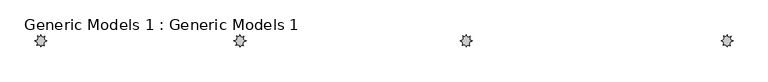
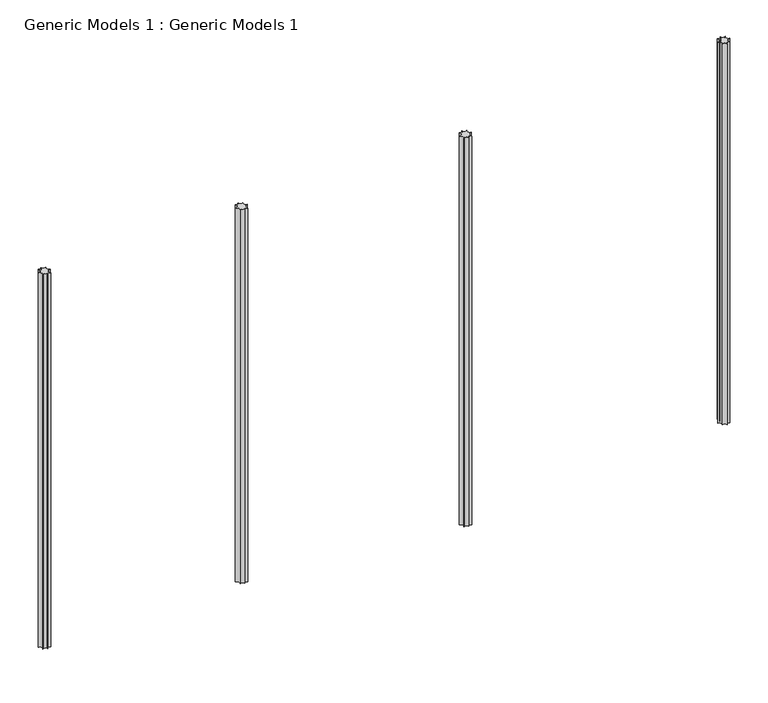
"""IFC4 building model written with IfcOpenShell, lengths in millimetres: proxy geometry, Generic Models 1 : Generic Models 1."""

from ifc_helpers import new_model, si_unit, frame, origin, place, context, project, spatial, polyline, circle_curve, source, transform, mapped, element, save
from ifc_brep_helpers import plane_surface, revolved_surface, advanced_brep


def generic_models_1_generic_models_1_27fef2d6(model_context):
    return source(origin(), model_context, "Body", "AdvancedBrep", [
        advanced_brep(
        [(-16868.2183666, -7371.697034, 6717.0608213), (-16912.6683666, -7455.6996381, 6717.0608213), (-16878.4321748, -7531.7567045, 6717.0608213), (-16811.0683666, -7557.2996381, 6717.0608213), (-16753.9183666, -7539.7022422, 6717.0608213), (-16709.4683666, -7455.6996381, 6717.0608213), (-16743.7045585, -7379.6425717, 6717.0608213), (-16811.0683666, -7354.0996381, 6717.0608213), (-16868.2183666, -7371.697034, 0.0), (-16811.0683666, -7354.0996381, 0.0), (-16743.7045585, -7379.6425717, 0.0), (-16709.4683666, -7455.6996381, 0.0), (-16753.9183666, -7539.7022422, 0.0), (-16811.0683666, -7557.2996381, 0.0), (-16878.4321748, -7531.7567045, 0.0), (-16912.6683666, -7455.6996381, 0.0)],
        [
            (0, 1, circle_curve(frame((-16912.6683666, -7401.9379714, 6717.0608213), z_axis=(0.0, 0.0, -1.0), x_axis=(1.0, 0.0, 0.0)), 53.7616666)),
            (1, 2, circle_curve(frame((-16912.6683666, -7501.4336804, 6717.0608213), z_axis=(0.0, 0.0, -1.0), x_axis=(1.0, 0.0, 0.0)), 45.7340423)),
            (2, 3, circle_curve(frame((-16849.5929412, -7557.2996381, 6717.0608213), z_axis=(0.0, 0.0, -1.0), x_axis=(1.0, 0.0, 0.0)), 38.5245746)),
            (3, 4, circle_curve(frame((-16779.7841073, -7557.2996381, 6717.0608213), z_axis=(0.0, 0.0, -1.0), x_axis=(1.0, 0.0, 0.0)), 31.2842593)),
            (4, 5, circle_curve(frame((-16709.4683666, -7509.4613047, 6717.0608213), z_axis=(0.0, 0.0, -1.0), x_axis=(1.0, 0.0, 0.0)), 53.7616666)),
            (5, 6, circle_curve(frame((-16709.4683666, -7409.9655958, 6717.0608213), z_axis=(0.0, 0.0, -1.0), x_axis=(1.0, 0.0, 0.0)), 45.7340423)),
            (6, 7, circle_curve(frame((-16772.543792, -7354.0996381, 6717.0608213), z_axis=(0.0, 0.0, -1.0), x_axis=(1.0, 0.0, 0.0)), 38.5245746)),
            (7, 0, circle_curve(frame((-16842.352626, -7354.0996381, 6717.0608213), z_axis=(0.0, 0.0, -1.0), x_axis=(1.0, 0.0, 0.0)), 31.2842593)),
            (8, 9, circle_curve(frame((-16842.352626, -7354.0996381, 0.0), z_axis=(0.0, 0.0, 1.0), x_axis=(1.0, 0.0, 0.0)), 31.2842593)),
            (9, 10, circle_curve(frame((-16772.543792, -7354.0996381, 0.0), z_axis=(0.0, 0.0, 1.0), x_axis=(1.0, 0.0, 0.0)), 38.5245746)),
            (10, 11, circle_curve(frame((-16709.4683666, -7409.9655958, 0.0), z_axis=(0.0, 0.0, 1.0), x_axis=(1.0, 0.0, 0.0)), 45.7340423)),
            (11, 12, circle_curve(frame((-16709.4683666, -7509.4613047, 0.0), z_axis=(0.0, 0.0, 1.0), x_axis=(1.0, 0.0, 0.0)), 53.7616666)),
            (12, 13, circle_curve(frame((-16779.7841073, -7557.2996381, 0.0), z_axis=(0.0, 0.0, 1.0), x_axis=(1.0, 0.0, 0.0)), 31.2842593)),
            (13, 14, circle_curve(frame((-16849.5929412, -7557.2996381, 0.0), z_axis=(0.0, 0.0, 1.0), x_axis=(1.0, 0.0, 0.0)), 38.5245746)),
            (14, 15, circle_curve(frame((-16912.6683666, -7501.4336804, 0.0), z_axis=(0.0, 0.0, 1.0), x_axis=(1.0, 0.0, 0.0)), 45.7340423)),
            (15, 8, circle_curve(frame((-16912.6683666, -7401.9379714, 0.0), z_axis=(0.0, 0.0, 1.0), x_axis=(1.0, 0.0, 0.0)), 53.7616666)),
            (0, 8),
            (15, 1),
            (14, 2),
            (13, 3),
            (12, 4),
            (11, 5),
            (10, 6),
            (9, 7),
        ],
        [
            plane_surface(frame((-16858.9067, -7401.9379714, 6717.0608213), z_axis=(0.0, 0.0, 1.0), x_axis=(0.0, -1.0, 0.0))),
            plane_surface(frame((-16858.9067, -7401.9379714, 0.0), z_axis=(0.0, 0.0, -1.0), x_axis=(0.0, 1.0, 0.0))),
            revolved_surface(polyline([(-16858.9067, -7401.9379714, 0.0), (-16858.9067, -7401.9379714, 6717.0608213)]), (-16912.6683666, -7401.9379714, 0.0), (0.0, 0.0, -1.0)),
            revolved_surface(polyline([(-16866.9343243, -7501.4336804, 0.0), (-16866.9343243, -7501.4336804, 6717.0608213)]), (-16912.6683666, -7501.4336804, 0.0), (0.0, 0.0, -1.0)),
            revolved_surface(polyline([(-16811.0683666, -7557.2996381, 0.0), (-16811.0683666, -7557.2996381, 6717.0608213)]), (-16849.5929412, -7557.2996381, 0.0), (0.0, 0.0, -1.0)),
            revolved_surface(polyline([(-16748.499848000003, -7557.2996381, 0.0), (-16748.499848000003, -7557.2996381, 6717.0608213)]), (-16779.7841073, -7557.2996381, 0.0), (0.0, 0.0, -1.0)),
            revolved_surface(polyline([(-16655.7067, -7509.4613047, 0.0), (-16655.7067, -7509.4613047, 6717.0608213)]), (-16709.4683666, -7509.4613047, 0.0), (0.0, 0.0, -1.0)),
            revolved_surface(polyline([(-16663.7343243, -7409.9655958, 0.0), (-16663.7343243, -7409.9655958, 6717.0608213)]), (-16709.4683666, -7409.9655958, 0.0), (0.0, 0.0, -1.0)),
            revolved_surface(polyline([(-16734.0192174, -7354.0996381, 0.0), (-16734.0192174, -7354.0996381, 6717.0608213)]), (-16772.543792, -7354.0996381, 0.0), (0.0, 0.0, -1.0)),
            revolved_surface(polyline([(-16811.0683667, -7354.0996381, 0.0), (-16811.0683667, -7354.0996381, 6717.0608213)]), (-16842.352626, -7354.0996381, 0.0), (0.0, 0.0, -1.0)),
        ],
        [
            (0, [[1, 2, 3, 4, 5, 6, 7, 8]]),
            (1, [[9, 10, 11, 12, 13, 14, 15, 16]]),
            (2, [[-1, 17, -16, 18]]),
            (3, [[-2, -18, -15, 19]]),
            (4, [[-3, -19, -14, 20]]),
            (5, [[-4, -20, -13, 21]]),
            (6, [[-5, -21, -12, 22]]),
            (7, [[-6, -22, -11, 23]]),
            (8, [[-7, -23, -10, 24]]),
            (9, [[-8, -24, -9, -17]]),
        ],
    ),
        advanced_brep(
        [(-13058.2183666, -7371.697034, 6680.2), (-13102.6683666, -7455.6996381, 6680.2), (-13068.4321748, -7531.7567045, 6680.2), (-13001.0683666, -7557.2996381, 6680.2), (-12943.9183666, -7539.7022422, 6680.2), (-12899.4683666, -7455.6996381, 6680.2), (-12933.7045585, -7379.6425717, 6680.2), (-13001.0683666, -7354.0996381, 6680.2), (-13058.2183666, -7371.697034, -309.3465665), (-13001.0683666, -7354.0996381, -309.3465665), (-12933.7045585, -7379.6425717, -309.3465665), (-12899.4683666, -7455.6996381, -309.3465665), (-12943.9183666, -7539.7022422, -309.3465665), (-13001.0683666, -7557.2996381, -309.3465665), (-13068.4321748, -7531.7567045, -309.3465665), (-13102.6683666, -7455.6996381, -309.3465665)],
        [
            (0, 1, circle_curve(frame((-13102.6683666, -7401.9379714, 6680.2), z_axis=(0.0, 0.0, -1.0), x_axis=(1.0, 0.0, 0.0)), 53.7616666)),
            (1, 2, circle_curve(frame((-13102.6683666, -7501.4336804, 6680.2), z_axis=(0.0, 0.0, -1.0), x_axis=(1.0, 0.0, 0.0)), 45.7340423)),
            (2, 3, circle_curve(frame((-13039.5929412, -7557.2996381, 6680.2), z_axis=(0.0, 0.0, -1.0), x_axis=(1.0, 0.0, 0.0)), 38.5245746)),
            (3, 4, circle_curve(frame((-12969.7841073, -7557.2996381, 6680.2), z_axis=(0.0, 0.0, -1.0), x_axis=(1.0, 0.0, 0.0)), 31.2842593)),
            (4, 5, circle_curve(frame((-12899.4683666, -7509.4613047, 6680.2), z_axis=(0.0, 0.0, -1.0), x_axis=(1.0, 0.0, 0.0)), 53.7616666)),
            (5, 6, circle_curve(frame((-12899.4683666, -7409.9655958, 6680.2), z_axis=(0.0, 0.0, -1.0), x_axis=(1.0, 0.0, 0.0)), 45.7340423)),
            (6, 7, circle_curve(frame((-12962.543792, -7354.0996381, 6680.2), z_axis=(0.0, 0.0, -1.0), x_axis=(1.0, 0.0, 0.0)), 38.5245746)),
            (7, 0, circle_curve(frame((-13032.352626, -7354.0996381, 6680.2), z_axis=(0.0, 0.0, -1.0), x_axis=(1.0, 0.0, 0.0)), 31.2842593)),
            (8, 9, circle_curve(frame((-13032.352626, -7354.0996381, -309.3465665), z_axis=(0.0, 0.0, 1.0), x_axis=(1.0, 0.0, 0.0)), 31.2842593)),
            (9, 10, circle_curve(frame((-12962.543792, -7354.0996381, -309.3465665), z_axis=(0.0, 0.0, 1.0), x_axis=(1.0, 0.0, 0.0)), 38.5245746)),
            (10, 11, circle_curve(frame((-12899.4683666, -7409.9655958, -309.3465665), z_axis=(0.0, 0.0, 1.0), x_axis=(1.0, 0.0, 0.0)), 45.7340423)),
            (11, 12, circle_curve(frame((-12899.4683666, -7509.4613047, -309.3465665), z_axis=(0.0, 0.0, 1.0), x_axis=(1.0, 0.0, 0.0)), 53.7616666)),
            (12, 13, circle_curve(frame((-12969.7841073, -7557.2996381, -309.3465665), z_axis=(0.0, 0.0, 1.0), x_axis=(1.0, 0.0, 0.0)), 31.2842593)),
            (13, 14, circle_curve(frame((-13039.5929412, -7557.2996381, -309.3465665), z_axis=(0.0, 0.0, 1.0), x_axis=(1.0, 0.0, 0.0)), 38.5245746)),
            (14, 15, circle_curve(frame((-13102.6683666, -7501.4336804, -309.3465665), z_axis=(0.0, 0.0, 1.0), x_axis=(1.0, 0.0, 0.0)), 45.7340423)),
            (15, 8, circle_curve(frame((-13102.6683666, -7401.9379714, -309.3465665), z_axis=(0.0, 0.0, 1.0), x_axis=(1.0, 0.0, 0.0)), 53.7616666)),
            (0, 8),
            (15, 1),
            (14, 2),
            (13, 3),
            (12, 4),
            (11, 5),
            (10, 6),
            (9, 7),
        ],
        [
            plane_surface(frame((-13048.9067, -7401.9379714, 6680.2), z_axis=(0.0, 0.0, 1.0), x_axis=(0.0, -1.0, 0.0))),
            plane_surface(frame((-13048.9067, -7401.9379714, -309.3465665), z_axis=(0.0, 0.0, -1.0), x_axis=(0.0, 1.0, 0.0))),
            revolved_surface(polyline([(-13048.906700000001, -7401.9379714, -309.3465665), (-13048.906700000001, -7401.9379714, 6680.2)]), (-13102.6683666, -7401.9379714, -309.3465665), (0.0, 0.0, -1.0)),
            revolved_surface(polyline([(-13056.9343243, -7501.4336804, -309.3465665), (-13056.9343243, -7501.4336804, 6680.2)]), (-13102.6683666, -7501.4336804, -309.3465665), (0.0, 0.0, -1.0)),
            revolved_surface(polyline([(-13001.0683666, -7557.2996381, -309.3465665), (-13001.0683666, -7557.2996381, 6680.2)]), (-13039.5929412, -7557.2996381, -309.3465665), (0.0, 0.0, -1.0)),
            revolved_surface(polyline([(-12938.499848, -7557.2996381, -309.3465665), (-12938.499848, -7557.2996381, 6680.2)]), (-12969.7841073, -7557.2996381, -309.3465665), (0.0, 0.0, -1.0)),
            revolved_surface(polyline([(-12845.7067, -7509.4613047, -309.3465665), (-12845.7067, -7509.4613047, 6680.2)]), (-12899.4683666, -7509.4613047, -309.3465665), (0.0, 0.0, -1.0)),
            revolved_surface(polyline([(-12853.7343243, -7409.9655958, -309.3465665), (-12853.7343243, -7409.9655958, 6680.2)]), (-12899.4683666, -7409.9655958, -309.3465665), (0.0, 0.0, -1.0)),
            revolved_surface(polyline([(-12924.0192174, -7354.0996381, -309.3465665), (-12924.0192174, -7354.0996381, 6680.2)]), (-12962.543792, -7354.0996381, -309.3465665), (0.0, 0.0, -1.0)),
            revolved_surface(polyline([(-13001.0683667, -7354.0996381, -309.3465665), (-13001.0683667, -7354.0996381, 6680.2)]), (-13032.352626, -7354.0996381, -309.3465665), (0.0, 0.0, -1.0)),
        ],
        [
            (0, [[1, 2, 3, 4, 5, 6, 7, 8]]),
            (1, [[9, 10, 11, 12, 13, 14, 15, 16]]),
            (2, [[-1, 17, -16, 18]]),
            (3, [[-2, -18, -15, 19]]),
            (4, [[-3, -19, -14, 20]]),
            (5, [[-4, -20, -13, 21]]),
            (6, [[-5, -21, -12, 22]]),
            (7, [[-6, -22, -11, 23]]),
            (8, [[-7, -23, -10, 24]]),
            (9, [[-8, -24, -9, -17]]),
        ],
    ),
        advanced_brep(
        [(-8664.0183666, -7371.697034, 6832.6), (-8708.4683666, -7455.6996381, 6832.6), (-8674.2321748, -7531.7567045, 6832.6), (-8606.8683666, -7557.2996381, 6832.6), (-8549.7183666, -7539.7022422, 6832.6), (-8505.2683666, -7455.6996381, 6832.6), (-8539.5045585, -7379.6425717, 6832.6), (-8606.8683666, -7354.0996381, 6832.6), (-8664.0183666, -7371.697034, -15.8978184), (-8606.8683666, -7354.0996381, -15.8978184), (-8539.5045585, -7379.6425717, -15.8978184), (-8505.2683666, -7455.6996381, -15.8978184), (-8549.7183666, -7539.7022422, -15.8978184), (-8606.8683666, -7557.2996381, -15.8978184), (-8674.2321748, -7531.7567045, -15.8978184), (-8708.4683666, -7455.6996381, -15.8978184)],
        [
            (0, 1, circle_curve(frame((-8708.4683666, -7401.9379714, 6832.6), z_axis=(0.0, 0.0, -1.0), x_axis=(1.0, 0.0, 0.0)), 53.7616666)),
            (1, 2, circle_curve(frame((-8708.4683666, -7501.4336804, 6832.6), z_axis=(0.0, 0.0, -1.0), x_axis=(1.0, 0.0, 0.0)), 45.7340423)),
            (2, 3, circle_curve(frame((-8645.3929412, -7557.2996381, 6832.6), z_axis=(0.0, 0.0, -1.0), x_axis=(1.0, 0.0, 0.0)), 38.5245746)),
            (3, 4, circle_curve(frame((-8575.5841073, -7557.2996381, 6832.6), z_axis=(0.0, 0.0, -1.0), x_axis=(1.0, 0.0, 0.0)), 31.2842593)),
            (4, 5, circle_curve(frame((-8505.2683666, -7509.4613047, 6832.6), z_axis=(0.0, 0.0, -1.0), x_axis=(1.0, 0.0, 0.0)), 53.7616666)),
            (5, 6, circle_curve(frame((-8505.2683666, -7409.9655958, 6832.6), z_axis=(0.0, 0.0, -1.0), x_axis=(1.0, 0.0, 0.0)), 45.7340423)),
            (6, 7, circle_curve(frame((-8568.343792, -7354.0996381, 6832.6), z_axis=(0.0, 0.0, -1.0), x_axis=(1.0, 0.0, 0.0)), 38.5245746)),
            (7, 0, circle_curve(frame((-8638.152626, -7354.0996381, 6832.6), z_axis=(0.0, 0.0, -1.0), x_axis=(1.0, 0.0, 0.0)), 31.2842593)),
            (8, 9, circle_curve(frame((-8638.152626, -7354.0996381, -15.8978184), z_axis=(0.0, 0.0, 1.0), x_axis=(1.0, 0.0, 0.0)), 31.2842593)),
            (9, 10, circle_curve(frame((-8568.343792, -7354.0996381, -15.8978184), z_axis=(0.0, 0.0, 1.0), x_axis=(1.0, 0.0, 0.0)), 38.5245746)),
            (10, 11, circle_curve(frame((-8505.2683666, -7409.9655958, -15.8978184), z_axis=(0.0, 0.0, 1.0), x_axis=(1.0, 0.0, 0.0)), 45.7340423)),
            (11, 12, circle_curve(frame((-8505.2683666, -7509.4613047, -15.8978184), z_axis=(0.0, 0.0, 1.0), x_axis=(1.0, 0.0, 0.0)), 53.7616666)),
            (12, 13, circle_curve(frame((-8575.5841073, -7557.2996381, -15.8978184), z_axis=(0.0, 0.0, 1.0), x_axis=(1.0, 0.0, 0.0)), 31.2842593)),
            (13, 14, circle_curve(frame((-8645.3929412, -7557.2996381, -15.8978184), z_axis=(0.0, 0.0, 1.0), x_axis=(1.0, 0.0, 0.0)), 38.5245746)),
            (14, 15, circle_curve(frame((-8708.4683666, -7501.4336804, -15.8978184), z_axis=(0.0, 0.0, 1.0), x_axis=(1.0, 0.0, 0.0)), 45.7340423)),
            (15, 8, circle_curve(frame((-8708.4683666, -7401.9379714, -15.8978184), z_axis=(0.0, 0.0, 1.0), x_axis=(1.0, 0.0, 0.0)), 53.7616666)),
            (0, 8),
            (15, 1),
            (14, 2),
            (13, 3),
            (12, 4),
            (11, 5),
            (10, 6),
            (9, 7),
        ],
        [
            plane_surface(frame((-8654.7067, -7401.9379714, 6832.6), z_axis=(0.0, 0.0, 1.0), x_axis=(0.0, -1.0, 0.0))),
            plane_surface(frame((-8654.7067, -7401.9379714, -15.8978184), z_axis=(0.0, 0.0, -1.0), x_axis=(0.0, 1.0, 0.0))),
            revolved_surface(polyline([(-8654.7067, -7401.9379714, -15.8978184), (-8654.7067, -7401.9379714, 6832.6)]), (-8708.4683666, -7401.9379714, -15.8978184), (0.0, 0.0, -1.0)),
            revolved_surface(polyline([(-8662.7343243, -7501.4336804, -15.8978184), (-8662.7343243, -7501.4336804, 6832.6)]), (-8708.4683666, -7501.4336804, -15.8978184), (0.0, 0.0, -1.0)),
            revolved_surface(polyline([(-8606.8683666, -7557.2996381, -15.8978184), (-8606.8683666, -7557.2996381, 6832.6)]), (-8645.3929412, -7557.2996381, -15.8978184), (0.0, 0.0, -1.0)),
            revolved_surface(polyline([(-8544.299847999999, -7557.2996381, -15.8978184), (-8544.299847999999, -7557.2996381, 6832.6)]), (-8575.5841073, -7557.2996381, -15.8978184), (0.0, 0.0, -1.0)),
            revolved_surface(polyline([(-8451.5067, -7509.4613047, -15.8978184), (-8451.5067, -7509.4613047, 6832.6)]), (-8505.2683666, -7509.4613047, -15.8978184), (0.0, 0.0, -1.0)),
            revolved_surface(polyline([(-8459.534324299999, -7409.9655958, -15.8978184), (-8459.534324299999, -7409.9655958, 6832.6)]), (-8505.2683666, -7409.9655958, -15.8978184), (0.0, 0.0, -1.0)),
            revolved_surface(polyline([(-8529.8192174, -7354.0996381, -15.8978184), (-8529.8192174, -7354.0996381, 6832.6)]), (-8568.343792, -7354.0996381, -15.8978184), (0.0, 0.0, -1.0)),
            revolved_surface(polyline([(-8606.868366699999, -7354.0996381, -15.8978184), (-8606.868366699999, -7354.0996381, 6832.6)]), (-8638.152626, -7354.0996381, -15.8978184), (0.0, 0.0, -1.0)),
        ],
        [
            (0, [[1, 2, 3, 4, 5, 6, 7, 8]]),
            (1, [[9, 10, 11, 12, 13, 14, 15, 16]]),
            (2, [[-1, 17, -16, 18]]),
            (3, [[-2, -18, -15, 19]]),
            (4, [[-3, -19, -14, 20]]),
            (5, [[-4, -20, -13, 21]]),
            (6, [[-5, -21, -12, 22]]),
            (7, [[-6, -22, -11, 23]]),
            (8, [[-7, -23, -10, 24]]),
            (9, [[-8, -24, -9, -17]]),
        ],
    ),
        advanced_brep(
        [(-20221.0183666, -7371.697034, 6729.0937292), (-20265.4683666, -7455.6996381, 6729.0937292), (-20231.2321748, -7531.7567045, 6729.0937292), (-20163.8683666, -7557.2996381, 6729.0937292), (-20106.7183666, -7539.7022422, 6729.0937292), (-20062.2683666, -7455.6996381, 6729.0937292), (-20096.5045585, -7379.6425717, 6729.0937292), (-20163.8683666, -7354.0996381, 6729.0937292), (-20221.0183666, -7371.697034, 0.0), (-20163.8683666, -7354.0996381, 0.0), (-20096.5045585, -7379.6425717, 0.0), (-20062.2683666, -7455.6996381, 0.0), (-20106.7183666, -7539.7022422, 0.0), (-20163.8683666, -7557.2996381, 0.0), (-20231.2321748, -7531.7567045, 0.0), (-20265.4683666, -7455.6996381, 0.0)],
        [
            (0, 1, circle_curve(frame((-20265.4683666, -7401.9379714, 6729.0937292), z_axis=(0.0, 0.0, -1.0), x_axis=(1.0, 0.0, 0.0)), 53.7616666)),
            (1, 2, circle_curve(frame((-20265.4683666, -7501.4336804, 6729.0937292), z_axis=(0.0, 0.0, -1.0), x_axis=(1.0, 0.0, 0.0)), 45.7340423)),
            (2, 3, circle_curve(frame((-20202.3929412, -7557.2996381, 6729.0937292), z_axis=(0.0, 0.0, -1.0), x_axis=(1.0, 0.0, 0.0)), 38.5245746)),
            (3, 4, circle_curve(frame((-20132.5841073, -7557.2996381, 6729.0937292), z_axis=(0.0, 0.0, -1.0), x_axis=(1.0, 0.0, 0.0)), 31.2842593)),
            (4, 5, circle_curve(frame((-20062.2683666, -7509.4613047, 6729.0937292), z_axis=(0.0, 0.0, -1.0), x_axis=(1.0, 0.0, 0.0)), 53.7616666)),
            (5, 6, circle_curve(frame((-20062.2683666, -7409.9655958, 6729.0937292), z_axis=(0.0, 0.0, -1.0), x_axis=(1.0, 0.0, 0.0)), 45.7340423)),
            (6, 7, circle_curve(frame((-20125.343792, -7354.0996381, 6729.0937292), z_axis=(0.0, 0.0, -1.0), x_axis=(1.0, 0.0, 0.0)), 38.5245746)),
            (7, 0, circle_curve(frame((-20195.152626, -7354.0996381, 6729.0937292), z_axis=(0.0, 0.0, -1.0), x_axis=(1.0, 0.0, 0.0)), 31.2842593)),
            (8, 9, circle_curve(frame((-20195.152626, -7354.0996381, 0.0), z_axis=(0.0, 0.0, 1.0), x_axis=(1.0, 0.0, 0.0)), 31.2842593)),
            (9, 10, circle_curve(frame((-20125.343792, -7354.0996381, 0.0), z_axis=(0.0, 0.0, 1.0), x_axis=(1.0, 0.0, 0.0)), 38.5245746)),
            (10, 11, circle_curve(frame((-20062.2683666, -7409.9655958, 0.0), z_axis=(0.0, 0.0, 1.0), x_axis=(1.0, 0.0, 0.0)), 45.7340423)),
            (11, 12, circle_curve(frame((-20062.2683666, -7509.4613047, 0.0), z_axis=(0.0, 0.0, 1.0), x_axis=(1.0, 0.0, 0.0)), 53.7616666)),
            (12, 13, circle_curve(frame((-20132.5841073, -7557.2996381, 0.0), z_axis=(0.0, 0.0, 1.0), x_axis=(1.0, 0.0, 0.0)), 31.2842593)),
            (13, 14, circle_curve(frame((-20202.3929412, -7557.2996381, 0.0), z_axis=(0.0, 0.0, 1.0), x_axis=(1.0, 0.0, 0.0)), 38.5245746)),
            (14, 15, circle_curve(frame((-20265.4683666, -7501.4336804, 0.0), z_axis=(0.0, 0.0, 1.0), x_axis=(1.0, 0.0, 0.0)), 45.7340423)),
            (15, 8, circle_curve(frame((-20265.4683666, -7401.9379714, 0.0), z_axis=(0.0, 0.0, 1.0), x_axis=(1.0, 0.0, 0.0)), 53.7616666)),
            (0, 8),
            (15, 1),
            (14, 2),
            (13, 3),
            (12, 4),
            (11, 5),
            (10, 6),
            (9, 7),
        ],
        [
            plane_surface(frame((-20211.7067, -7401.9379714, 6729.0937292), z_axis=(0.0, 0.0, 1.0), x_axis=(0.0, -1.0, 0.0))),
            plane_surface(frame((-20211.7067, -7401.9379714, 0.0), z_axis=(0.0, 0.0, -1.0), x_axis=(0.0, 1.0, 0.0))),
            revolved_surface(polyline([(-20211.7067, -7401.9379714, 0.0), (-20211.7067, -7401.9379714, 6729.0937292)]), (-20265.4683666, -7401.9379714, 0.0), (0.0, 0.0, -1.0)),
            revolved_surface(polyline([(-20219.7343243, -7501.4336804, 0.0), (-20219.7343243, -7501.4336804, 6729.0937292)]), (-20265.4683666, -7501.4336804, 0.0), (0.0, 0.0, -1.0)),
            revolved_surface(polyline([(-20163.8683666, -7557.2996381, 0.0), (-20163.8683666, -7557.2996381, 6729.0937292)]), (-20202.3929412, -7557.2996381, 0.0), (0.0, 0.0, -1.0)),
            revolved_surface(polyline([(-20101.299848000002, -7557.2996381, 0.0), (-20101.299848000002, -7557.2996381, 6729.0937292)]), (-20132.5841073, -7557.2996381, 0.0), (0.0, 0.0, -1.0)),
            revolved_surface(polyline([(-20008.5067, -7509.4613047, 0.0), (-20008.5067, -7509.4613047, 6729.0937292)]), (-20062.2683666, -7509.4613047, 0.0), (0.0, 0.0, -1.0)),
            revolved_surface(polyline([(-20016.534324300002, -7409.9655958, 0.0), (-20016.534324300002, -7409.9655958, 6729.0937292)]), (-20062.2683666, -7409.9655958, 0.0), (0.0, 0.0, -1.0)),
            revolved_surface(polyline([(-20086.8192174, -7354.0996381, 0.0), (-20086.8192174, -7354.0996381, 6729.0937292)]), (-20125.343792, -7354.0996381, 0.0), (0.0, 0.0, -1.0)),
            revolved_surface(polyline([(-20163.8683667, -7354.0996381, 0.0), (-20163.8683667, -7354.0996381, 6729.0937292)]), (-20195.152626, -7354.0996381, 0.0), (0.0, 0.0, -1.0)),
        ],
        [
            (0, [[1, 2, 3, 4, 5, 6, 7, 8]]),
            (1, [[9, 10, 11, 12, 13, 14, 15, 16]]),
            (2, [[-1, 17, -16, 18]]),
            (3, [[-2, -18, -15, 19]]),
            (4, [[-3, -19, -14, 20]]),
            (5, [[-4, -20, -13, 21]]),
            (6, [[-5, -21, -12, 22]]),
            (7, [[-6, -22, -11, 23]]),
            (8, [[-7, -23, -10, 24]]),
            (9, [[-8, -24, -9, -17]]),
        ],
    ),
    ])


if __name__ == "__main__":
    model = new_model("IFC4")
    model_context = context("Model", 3, world=origin())
    ifc_project = project(units=[si_unit("LENGTHUNIT", "METRE", prefix="MILLI")], contexts=[model_context])
    site = spatial("IfcSite", under=ifc_project)
    building = spatial("IfcBuilding", under=site)
    placement = place(None, origin())
    generic_models_1_generic_models_1_shape = generic_models_1_generic_models_1_27fef2d6(model_context)
    element("IfcBuildingElementProxy", 1, Name="Generic Models 1 : Generic Models 1", ObjectType="Generic Models 1 : Generic Models 1", at=placement, inside=building, context=model_context, shape_type="MappedRepresentation", body=[
        mapped(generic_models_1_generic_models_1_shape, transform((0.0, 0.0, 0.0), x_axis=(1.0, 0.0, 0.0), y_axis=(0.0, 1.0, 0.0), z_axis=(0.0, 0.0, 1.0))),
    ])
    save(model, "model.ifc")
